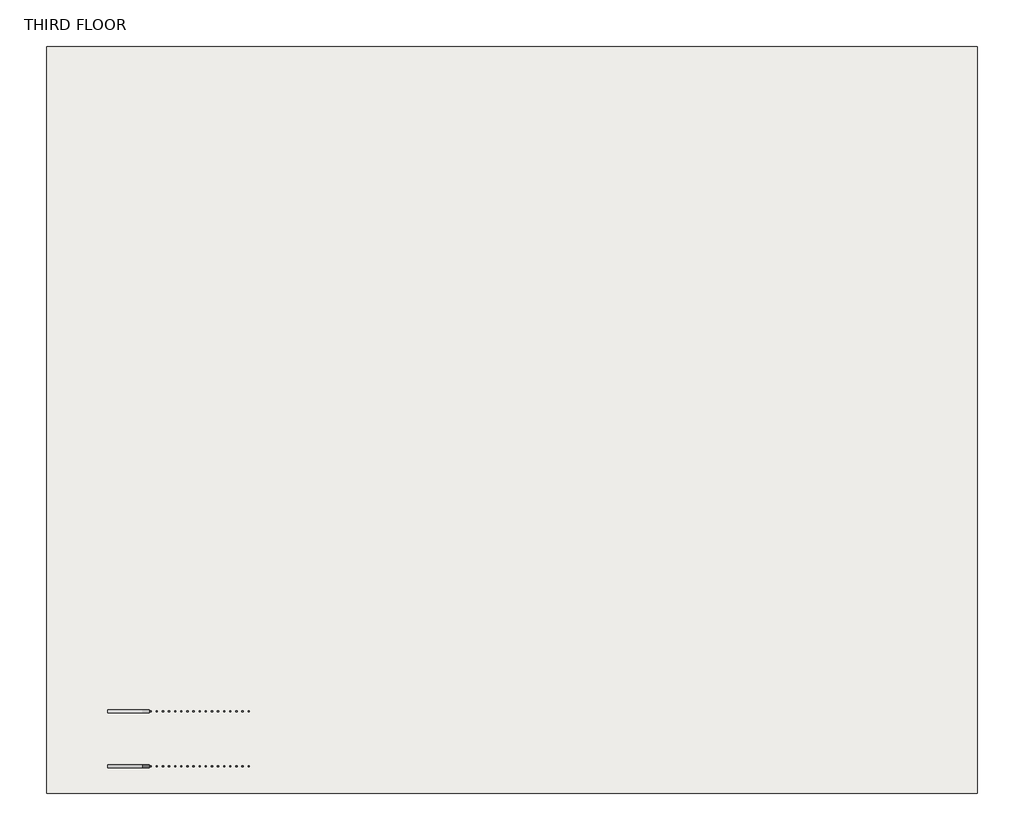
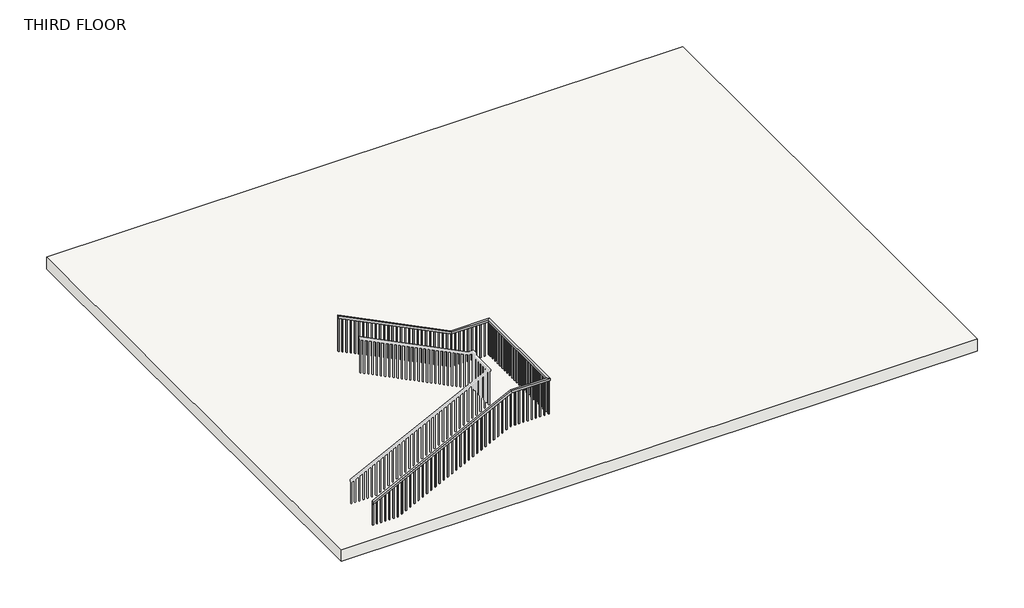
# One storey, part 1 of 2: 1 railing, 1 slab.
"""IFC4 building model written with IfcOpenShell, lengths in millimetres."""

from ifc_helpers import new_model, si_unit, frame, origin, place, context, project, spatial, polyline, outline, extrude, faceted_brep, element, save

model = new_model("IFC4")

# Units and contexts
model_context = context("Model", 3, world=origin())
ifc_project = project(units=[si_unit("LENGTHUNIT", "METRE", prefix="MILLI")], contexts=[model_context])

# Site, building, storey
site = spatial("IfcSite", under=ifc_project)
building = spatial("IfcBuilding", under=site)
storey = spatial("IfcBuildingStorey", under=building, Name="THIRD FLOOR", Elevation=9144.0)

# Railing
placement = place(None, origin())
element("IfcRailing", 1, ObjectType="Handrail - Rectangular", at=placement, inside=storey, context=model_context, shape_type="SolidModel", body=[
    faceted_brep([(-8362.2800418, -5370.1090076, 10058.4), (-8362.2800418, -5370.1090076, 10001.6038734), (-8362.2800418, -5420.9090076, 10001.6038734), (-8362.2800418, -5420.9090076, 10058.4), (-5009.4800418, -5370.1090076, 11734.8), (-4997.4877885, -5370.1090076, 11684.0), (-4997.4877885, -5420.9090076, 11684.0), (-5009.4800418, -5420.9090076, 11734.8), (-4120.4800418, -5370.1090076, 11734.8), (-4120.4800418, -5370.1090076, 11684.0), (-4069.6800418, -5420.9090076, 11684.0), (-4069.6800418, -5420.9090076, 11734.8), (-4120.4800418, -2917.1346494, 11734.8), (-4120.4800418, -2917.1346494, 11684.0), (-4069.6800418, -2866.3346494, 11684.0), (-4069.6800418, -2866.3346494, 11734.8), (-5009.4800418, -2917.1346494, 11734.8), (-5021.472295, -2917.1346494, 11684.0), (-5021.472295, -2866.3346494, 11684.0), (-5009.4800418, -2866.3346494, 11734.8), (-7752.6800418, -2917.1346494, 13106.4), (-7752.6800418, -2866.3346494, 13106.4), (-7752.6800418, -2866.3346494, 13049.6038734), (-7752.6800418, -2917.1346494, 13049.6038734)], [[[0, 1, 2, 3]], [[1, 0, 4, 5]], [[2, 1, 5, 6]], [[3, 2, 6, 7]], [[0, 3, 7, 4]], [[5, 4, 8, 9]], [[6, 5, 9, 10]], [[7, 6, 10, 11]], [[4, 7, 11, 8]], [[9, 8, 12, 13]], [[10, 9, 13, 14]], [[11, 10, 14, 15]], [[8, 11, 15, 12]], [[13, 12, 16, 17]], [[14, 13, 17, 18]], [[15, 14, 18, 19]], [[12, 15, 19, 16]], [[20, 21, 22, 23]], [[17, 16, 20, 23]], [[18, 17, 23, 22]], [[19, 18, 22, 21]], [[16, 19, 21, 20]]]),
    extrude(outline(polyline([(13003.5663734, -7660.6050418), (12145.9625, -7660.6050418), (12136.4375, -7641.5550418), (12994.0413734, -7641.5550418), (13003.5663734, -7660.6050418)])), frame((0.0, -2901.2596494, 0.0), z_axis=(0.0, 1.0, 0.0), x_axis=(0.0, 0.0, 1.0)), (0.0, 0.0, 1.0), 19.05),
    extrude(outline(polyline([(12952.7663734, -7559.0050418), (12095.1625, -7559.0050418), (12085.6375, -7539.9550418), (12943.2413734, -7539.9550418), (12952.7663734, -7559.0050418)])), frame((0.0, -2901.2596494, 0.0), z_axis=(0.0, 1.0, 0.0), x_axis=(0.0, 0.0, 1.0)), (0.0, 0.0, 1.0), 19.05),
    extrude(outline(polyline([(12901.9663734, -7457.4050418), (12044.3625, -7457.4050418), (12034.8375, -7438.3550418), (12892.4413734, -7438.3550418), (12901.9663734, -7457.4050418)])), frame((0.0, -2901.2596494, 0.0), z_axis=(0.0, 1.0, 0.0), x_axis=(0.0, 0.0, 1.0)), (0.0, 0.0, 1.0), 19.05),
    extrude(outline(polyline([(12851.1663734, -7355.8050418), (11993.5625, -7355.8050418), (11984.0375, -7336.7550418), (12841.6413734, -7336.7550418), (12851.1663734, -7355.8050418)])), frame((0.0, -2901.2596494, 0.0), z_axis=(0.0, 1.0, 0.0), x_axis=(0.0, 0.0, 1.0)), (0.0, 0.0, 1.0), 19.05),
    extrude(outline(polyline([(12800.3663734, -7254.2050418), (11942.7625, -7254.2050418), (11933.2375, -7235.1550418), (12790.8413734, -7235.1550418), (12800.3663734, -7254.2050418)])), frame((0.0, -2901.2596494, 0.0), z_axis=(0.0, 1.0, 0.0), x_axis=(0.0, 0.0, 1.0)), (0.0, 0.0, 1.0), 19.05),
    extrude(outline(polyline([(12749.5663734, -7152.6050418), (11891.9625, -7152.6050418), (11882.4375, -7133.5550418), (12740.0413734, -7133.5550418), (12749.5663734, -7152.6050418)])), frame((0.0, -2901.2596494, 0.0), z_axis=(0.0, 1.0, 0.0), x_axis=(0.0, 0.0, 1.0)), (0.0, 0.0, 1.0), 19.05),
    extrude(outline(polyline([(12698.7663734, -7051.0050418), (11841.1625, -7051.0050418), (11831.6375, -7031.9550418), (12689.2413734, -7031.9550418), (12698.7663734, -7051.0050418)])), frame((0.0, -2901.2596494, 0.0), z_axis=(0.0, 1.0, 0.0), x_axis=(0.0, 0.0, 1.0)), (0.0, 0.0, 1.0), 19.05),
    extrude(outline(polyline([(12647.9663734, -6949.4050418), (11790.3625, -6949.4050418), (11780.8375, -6930.3550418), (12638.4413734, -6930.3550418), (12647.9663734, -6949.4050418)])), frame((0.0, -2901.2596494, 0.0), z_axis=(0.0, 1.0, 0.0), x_axis=(0.0, 0.0, 1.0)), (0.0, 0.0, 1.0), 19.05),
    extrude(outline(polyline([(12597.1663734, -6847.8050418), (11739.5625, -6847.8050418), (11730.0375, -6828.7550418), (12587.6413734, -6828.7550418), (12597.1663734, -6847.8050418)])), frame((0.0, -2901.2596494, 0.0), z_axis=(0.0, 1.0, 0.0), x_axis=(0.0, 0.0, 1.0)), (0.0, 0.0, 1.0), 19.05),
    extrude(outline(polyline([(12546.3663734, -6746.2050418), (11688.7625, -6746.2050418), (11679.2375, -6727.1550418), (12536.8413734, -6727.1550418), (12546.3663734, -6746.2050418)])), frame((0.0, -2901.2596494, 0.0), z_axis=(0.0, 1.0, 0.0), x_axis=(0.0, 0.0, 1.0)), (0.0, 0.0, 1.0), 19.05),
    extrude(outline(polyline([(12495.5663734, -6644.6050418), (11637.9625, -6644.6050418), (11628.4375, -6625.5550418), (12486.0413734, -6625.5550418), (12495.5663734, -6644.6050418)])), frame((0.0, -2901.2596494, 0.0), z_axis=(0.0, 1.0, 0.0), x_axis=(0.0, 0.0, 1.0)), (0.0, 0.0, 1.0), 19.05),
    extrude(outline(polyline([(12444.7663734, -6543.0050418), (11587.1625, -6543.0050418), (11577.6375, -6523.9550418), (12435.2413734, -6523.9550418), (12444.7663734, -6543.0050418)])), frame((0.0, -2901.2596494, 0.0), z_axis=(0.0, 1.0, 0.0), x_axis=(0.0, 0.0, 1.0)), (0.0, 0.0, 1.0), 19.05),
    extrude(outline(polyline([(12393.9663734, -6441.4050418), (11536.3625, -6441.4050418), (11526.8375, -6422.3550418), (12384.4413734, -6422.3550418), (12393.9663734, -6441.4050418)])), frame((0.0, -2901.2596494, 0.0), z_axis=(0.0, 1.0, 0.0), x_axis=(0.0, 0.0, 1.0)), (0.0, 0.0, 1.0), 19.05),
    extrude(outline(polyline([(12343.1663734, -6339.8050418), (11485.5625, -6339.8050418), (11476.0375, -6320.7550418), (12333.6413734, -6320.7550418), (12343.1663734, -6339.8050418)])), frame((0.0, -2901.2596494, 0.0), z_axis=(0.0, 1.0, 0.0), x_axis=(0.0, 0.0, 1.0)), (0.0, 0.0, 1.0), 19.05),
    extrude(outline(polyline([(12292.3663734, -6238.2050418), (11434.7625, -6238.2050418), (11425.2375, -6219.1550418), (12282.8413734, -6219.1550418), (12292.3663734, -6238.2050418)])), frame((0.0, -2901.2596494, 0.0), z_axis=(0.0, 1.0, 0.0), x_axis=(0.0, 0.0, 1.0)), (0.0, 0.0, 1.0), 19.05),
    extrude(outline(polyline([(12241.5663734, -6136.6050418), (11383.9625, -6136.6050418), (11374.4375, -6117.5550418), (12232.0413734, -6117.5550418), (12241.5663734, -6136.6050418)])), frame((0.0, -2901.2596494, 0.0), z_axis=(0.0, 1.0, 0.0), x_axis=(0.0, 0.0, 1.0)), (0.0, 0.0, 1.0), 19.05),
    extrude(outline(polyline([(12190.7663734, -6035.0050418), (11333.1625, -6035.0050418), (11323.6375, -6015.9550418), (12181.2413734, -6015.9550418), (12190.7663734, -6035.0050418)])), frame((0.0, -2901.2596494, 0.0), z_axis=(0.0, 1.0, 0.0), x_axis=(0.0, 0.0, 1.0)), (0.0, 0.0, 1.0), 19.05),
    extrude(outline(polyline([(12139.9663734, -5933.4050418), (11282.3625, -5933.4050418), (11272.8375, -5914.3550418), (12130.4413734, -5914.3550418), (12139.9663734, -5933.4050418)])), frame((0.0, -2901.2596494, 0.0), z_axis=(0.0, 1.0, 0.0), x_axis=(0.0, 0.0, 1.0)), (0.0, 0.0, 1.0), 19.05),
    extrude(outline(polyline([(12089.1663734, -5831.8050418), (11231.5625, -5831.8050418), (11222.0375, -5812.7550418), (12079.6413734, -5812.7550418), (12089.1663734, -5831.8050418)])), frame((0.0, -2901.2596494, 0.0), z_axis=(0.0, 1.0, 0.0), x_axis=(0.0, 0.0, 1.0)), (0.0, 0.0, 1.0), 19.05),
    extrude(outline(polyline([(12038.3663734, -5730.2050418), (11180.7625, -5730.2050418), (11171.2375, -5711.1550418), (12028.8413734, -5711.1550418), (12038.3663734, -5730.2050418)])), frame((0.0, -2901.2596494, 0.0), z_axis=(0.0, 1.0, 0.0), x_axis=(0.0, 0.0, 1.0)), (0.0, 0.0, 1.0), 19.05),
    extrude(outline(polyline([(11987.5663734, -5628.6050418), (11129.9625, -5628.6050418), (11120.4375, -5609.5550418), (11978.0413734, -5609.5550418), (11987.5663734, -5628.6050418)])), frame((0.0, -2901.2596494, 0.0), z_axis=(0.0, 1.0, 0.0), x_axis=(0.0, 0.0, 1.0)), (0.0, 0.0, 1.0), 19.05),
    extrude(outline(polyline([(11936.7663734, -5527.0050418), (11079.1625, -5527.0050418), (11069.6375, -5507.9550418), (11927.2413734, -5507.9550418), (11936.7663734, -5527.0050418)])), frame((0.0, -2901.2596494, 0.0), z_axis=(0.0, 1.0, 0.0), x_axis=(0.0, 0.0, 1.0)), (0.0, 0.0, 1.0), 19.05),
    extrude(outline(polyline([(11885.9663734, -5425.4050418), (11028.3625, -5425.4050418), (11018.8375, -5406.3550418), (11876.4413734, -5406.3550418), (11885.9663734, -5425.4050418)])), frame((0.0, -2901.2596494, 0.0), z_axis=(0.0, 1.0, 0.0), x_axis=(0.0, 0.0, 1.0)), (0.0, 0.0, 1.0), 19.05),
    extrude(outline(polyline([(11835.1663734, -5323.8050418), (10977.5625, -5323.8050418), (10968.0375, -5304.7550418), (11825.6413734, -5304.7550418), (11835.1663734, -5323.8050418)])), frame((0.0, -2901.2596494, 0.0), z_axis=(0.0, 1.0, 0.0), x_axis=(0.0, 0.0, 1.0)), (0.0, 0.0, 1.0), 19.05),
    extrude(outline(polyline([(11784.3663734, -5222.2050418), (10926.7625, -5222.2050418), (10917.2375, -5203.1550418), (11774.8413734, -5203.1550418), (11784.3663734, -5222.2050418)])), frame((0.0, -2901.2596494, 0.0), z_axis=(0.0, 1.0, 0.0), x_axis=(0.0, 0.0, 1.0)), (0.0, 0.0, 1.0), 19.05),
    extrude(outline(polyline([(11733.5663734, -5120.6050418), (10875.9625, -5120.6050418), (10866.4375, -5101.5550418), (11724.0413734, -5101.5550418), (11733.5663734, -5120.6050418)])), frame((0.0, -2901.2596494, 0.0), z_axis=(0.0, 1.0, 0.0), x_axis=(0.0, 0.0, 1.0)), (0.0, 0.0, 1.0), 19.05),
    extrude(outline(polyline([(-4898.3550418, -2901.2596494), (-4917.4050418, -2901.2596494), (-4917.4050418, -2882.2096494), (-4898.3550418, -2882.2096494), (-4898.3550418, -2901.2596494)])), frame((0.0, 0.0, 10820.4), z_axis=(0.0, 0.0, 1.0), x_axis=(1.0, 0.0, 0.0)), (0.0, 0.0, 1.0), 863.6),
    extrude(outline(polyline([(-4796.7550418, -2901.2596494), (-4815.8050418, -2901.2596494), (-4815.8050418, -2882.2096494), (-4796.7550418, -2882.2096494), (-4796.7550418, -2901.2596494)])), frame((0.0, 0.0, 10820.4), z_axis=(0.0, 0.0, 1.0), x_axis=(1.0, 0.0, 0.0)), (0.0, 0.0, 1.0), 863.6),
    extrude(outline(polyline([(-4695.1550418, -2901.2596494), (-4714.2050418, -2901.2596494), (-4714.2050418, -2882.2096494), (-4695.1550418, -2882.2096494), (-4695.1550418, -2901.2596494)])), frame((0.0, 0.0, 10820.4), z_axis=(0.0, 0.0, 1.0), x_axis=(1.0, 0.0, 0.0)), (0.0, 0.0, 1.0), 863.6),
    extrude(outline(polyline([(-4593.5550418, -2901.2596494), (-4612.6050418, -2901.2596494), (-4612.6050418, -2882.2096494), (-4593.5550418, -2882.2096494), (-4593.5550418, -2901.2596494)])), frame((0.0, 0.0, 10820.4), z_axis=(0.0, 0.0, 1.0), x_axis=(1.0, 0.0, 0.0)), (0.0, 0.0, 1.0), 863.6),
    extrude(outline(polyline([(-4491.9550418, -2901.2596494), (-4511.0050418, -2901.2596494), (-4511.0050418, -2882.2096494), (-4491.9550418, -2882.2096494), (-4491.9550418, -2901.2596494)])), frame((0.0, 0.0, 10820.4), z_axis=(0.0, 0.0, 1.0), x_axis=(1.0, 0.0, 0.0)), (0.0, 0.0, 1.0), 863.6),
    extrude(outline(polyline([(-4390.3550418, -2901.2596494), (-4409.4050418, -2901.2596494), (-4409.4050418, -2882.2096494), (-4390.3550418, -2882.2096494), (-4390.3550418, -2901.2596494)])), frame((0.0, 0.0, 10820.4), z_axis=(0.0, 0.0, 1.0), x_axis=(1.0, 0.0, 0.0)), (0.0, 0.0, 1.0), 863.6),
    extrude(outline(polyline([(-4288.7550418, -2901.2596494), (-4307.8050418, -2901.2596494), (-4307.8050418, -2882.2096494), (-4288.7550418, -2882.2096494), (-4288.7550418, -2901.2596494)])), frame((0.0, 0.0, 10820.4), z_axis=(0.0, 0.0, 1.0), x_axis=(1.0, 0.0, 0.0)), (0.0, 0.0, 1.0), 863.6),
    extrude(outline(polyline([(-4187.1550418, -2901.2596494), (-4206.2050418, -2901.2596494), (-4206.2050418, -2882.2096494), (-4187.1550418, -2882.2096494), (-4187.1550418, -2901.2596494)])), frame((0.0, 0.0, 10820.4), z_axis=(0.0, 0.0, 1.0), x_axis=(1.0, 0.0, 0.0)), (0.0, 0.0, 1.0), 863.6),
    extrude(outline(polyline([(-4104.6050418, -2966.6340076), (-4104.6050418, -2947.5840076), (-4085.5550418, -2947.5840076), (-4085.5550418, -2966.6340076), (-4104.6050418, -2966.6340076)])), frame((0.0, 0.0, 10820.4), z_axis=(0.0, 0.0, 1.0), x_axis=(1.0, 0.0, 0.0)), (0.0, 0.0, 1.0), 863.6),
    extrude(outline(polyline([(-4104.6050418, -3068.2340076), (-4104.6050418, -3049.1840076), (-4085.5550418, -3049.1840076), (-4085.5550418, -3068.2340076), (-4104.6050418, -3068.2340076)])), frame((0.0, 0.0, 10820.4), z_axis=(0.0, 0.0, 1.0), x_axis=(1.0, 0.0, 0.0)), (0.0, 0.0, 1.0), 863.6),
    extrude(outline(polyline([(-4104.6050418, -3169.8340076), (-4104.6050418, -3150.7840076), (-4085.5550418, -3150.7840076), (-4085.5550418, -3169.8340076), (-4104.6050418, -3169.8340076)])), frame((0.0, 0.0, 10820.4), z_axis=(0.0, 0.0, 1.0), x_axis=(1.0, 0.0, 0.0)), (0.0, 0.0, 1.0), 863.6),
    extrude(outline(polyline([(-4104.6050418, -3271.4340076), (-4104.6050418, -3252.3840076), (-4085.5550418, -3252.3840076), (-4085.5550418, -3271.4340076), (-4104.6050418, -3271.4340076)])), frame((0.0, 0.0, 10820.4), z_axis=(0.0, 0.0, 1.0), x_axis=(1.0, 0.0, 0.0)), (0.0, 0.0, 1.0), 863.6),
    extrude(outline(polyline([(-4104.6050418, -3373.0340076), (-4104.6050418, -3353.9840076), (-4085.5550418, -3353.9840076), (-4085.5550418, -3373.0340076), (-4104.6050418, -3373.0340076)])), frame((0.0, 0.0, 10820.4), z_axis=(0.0, 0.0, 1.0), x_axis=(1.0, 0.0, 0.0)), (0.0, 0.0, 1.0), 863.6),
    extrude(outline(polyline([(-4104.6050418, -3474.6340076), (-4104.6050418, -3455.5840076), (-4085.5550418, -3455.5840076), (-4085.5550418, -3474.6340076), (-4104.6050418, -3474.6340076)])), frame((0.0, 0.0, 10820.4), z_axis=(0.0, 0.0, 1.0), x_axis=(1.0, 0.0, 0.0)), (0.0, 0.0, 1.0), 863.6),
    extrude(outline(polyline([(-4104.6050418, -3576.2340076), (-4104.6050418, -3557.1840076), (-4085.5550418, -3557.1840076), (-4085.5550418, -3576.2340076), (-4104.6050418, -3576.2340076)])), frame((0.0, 0.0, 10820.4), z_axis=(0.0, 0.0, 1.0), x_axis=(1.0, 0.0, 0.0)), (0.0, 0.0, 1.0), 863.6),
    extrude(outline(polyline([(-4104.6050418, -3677.8340076), (-4104.6050418, -3658.7840076), (-4085.5550418, -3658.7840076), (-4085.5550418, -3677.8340076), (-4104.6050418, -3677.8340076)])), frame((0.0, 0.0, 10820.4), z_axis=(0.0, 0.0, 1.0), x_axis=(1.0, 0.0, 0.0)), (0.0, 0.0, 1.0), 863.6),
    extrude(outline(polyline([(-4104.6050418, -3779.4340076), (-4104.6050418, -3760.3840076), (-4085.5550418, -3760.3840076), (-4085.5550418, -3779.4340076), (-4104.6050418, -3779.4340076)])), frame((0.0, 0.0, 10820.4), z_axis=(0.0, 0.0, 1.0), x_axis=(1.0, 0.0, 0.0)), (0.0, 0.0, 1.0), 863.6),
    extrude(outline(polyline([(-4104.6050418, -3881.0340076), (-4104.6050418, -3861.9840076), (-4085.5550418, -3861.9840076), (-4085.5550418, -3881.0340076), (-4104.6050418, -3881.0340076)])), frame((0.0, 0.0, 10820.4), z_axis=(0.0, 0.0, 1.0), x_axis=(1.0, 0.0, 0.0)), (0.0, 0.0, 1.0), 863.6),
    extrude(outline(polyline([(-4104.6050418, -3982.6340076), (-4104.6050418, -3963.5840076), (-4085.5550418, -3963.5840076), (-4085.5550418, -3982.6340076), (-4104.6050418, -3982.6340076)])), frame((0.0, 0.0, 10820.4), z_axis=(0.0, 0.0, 1.0), x_axis=(1.0, 0.0, 0.0)), (0.0, 0.0, 1.0), 863.6),
    extrude(outline(polyline([(-4104.6050418, -4084.2340076), (-4104.6050418, -4065.1840076), (-4085.5550418, -4065.1840076), (-4085.5550418, -4084.2340076), (-4104.6050418, -4084.2340076)])), frame((0.0, 0.0, 10820.4), z_axis=(0.0, 0.0, 1.0), x_axis=(1.0, 0.0, 0.0)), (0.0, 0.0, 1.0), 863.6),
    extrude(outline(polyline([(-4104.6050418, -4185.8340076), (-4104.6050418, -4166.7840076), (-4085.5550418, -4166.7840076), (-4085.5550418, -4185.8340076), (-4104.6050418, -4185.8340076)])), frame((0.0, 0.0, 10820.4), z_axis=(0.0, 0.0, 1.0), x_axis=(1.0, 0.0, 0.0)), (0.0, 0.0, 1.0), 863.6),
    extrude(outline(polyline([(-4104.6050418, -4287.4340076), (-4104.6050418, -4268.3840076), (-4085.5550418, -4268.3840076), (-4085.5550418, -4287.4340076), (-4104.6050418, -4287.4340076)])), frame((0.0, 0.0, 10820.4), z_axis=(0.0, 0.0, 1.0), x_axis=(1.0, 0.0, 0.0)), (0.0, 0.0, 1.0), 863.6),
    extrude(outline(polyline([(-4104.6050418, -4389.0340076), (-4104.6050418, -4369.9840076), (-4085.5550418, -4369.9840076), (-4085.5550418, -4389.0340076), (-4104.6050418, -4389.0340076)])), frame((0.0, 0.0, 10820.4), z_axis=(0.0, 0.0, 1.0), x_axis=(1.0, 0.0, 0.0)), (0.0, 0.0, 1.0), 863.6),
    extrude(outline(polyline([(-4104.6050418, -4490.6340076), (-4104.6050418, -4471.5840076), (-4085.5550418, -4471.5840076), (-4085.5550418, -4490.6340076), (-4104.6050418, -4490.6340076)])), frame((0.0, 0.0, 10820.4), z_axis=(0.0, 0.0, 1.0), x_axis=(1.0, 0.0, 0.0)), (0.0, 0.0, 1.0), 863.6),
    extrude(outline(polyline([(-4104.6050418, -4592.2340076), (-4104.6050418, -4573.1840076), (-4085.5550418, -4573.1840076), (-4085.5550418, -4592.2340076), (-4104.6050418, -4592.2340076)])), frame((0.0, 0.0, 10820.4), z_axis=(0.0, 0.0, 1.0), x_axis=(1.0, 0.0, 0.0)), (0.0, 0.0, 1.0), 863.6),
    extrude(outline(polyline([(-4104.6050418, -4693.8340076), (-4104.6050418, -4674.7840076), (-4085.5550418, -4674.7840076), (-4085.5550418, -4693.8340076), (-4104.6050418, -4693.8340076)])), frame((0.0, 0.0, 10820.4), z_axis=(0.0, 0.0, 1.0), x_axis=(1.0, 0.0, 0.0)), (0.0, 0.0, 1.0), 863.6),
    extrude(outline(polyline([(-4104.6050418, -4795.4340076), (-4104.6050418, -4776.3840076), (-4085.5550418, -4776.3840076), (-4085.5550418, -4795.4340076), (-4104.6050418, -4795.4340076)])), frame((0.0, 0.0, 10820.4), z_axis=(0.0, 0.0, 1.0), x_axis=(1.0, 0.0, 0.0)), (0.0, 0.0, 1.0), 863.6),
    extrude(outline(polyline([(-4104.6050418, -4897.0340076), (-4104.6050418, -4877.9840076), (-4085.5550418, -4877.9840076), (-4085.5550418, -4897.0340076), (-4104.6050418, -4897.0340076)])), frame((0.0, 0.0, 10820.4), z_axis=(0.0, 0.0, 1.0), x_axis=(1.0, 0.0, 0.0)), (0.0, 0.0, 1.0), 863.6),
    extrude(outline(polyline([(-4104.6050418, -4998.6340076), (-4104.6050418, -4979.5840076), (-4085.5550418, -4979.5840076), (-4085.5550418, -4998.6340076), (-4104.6050418, -4998.6340076)])), frame((0.0, 0.0, 10820.4), z_axis=(0.0, 0.0, 1.0), x_axis=(1.0, 0.0, 0.0)), (0.0, 0.0, 1.0), 863.6),
    extrude(outline(polyline([(-4104.6050418, -5100.2340076), (-4104.6050418, -5081.1840076), (-4085.5550418, -5081.1840076), (-4085.5550418, -5100.2340076), (-4104.6050418, -5100.2340076)])), frame((0.0, 0.0, 10820.4), z_axis=(0.0, 0.0, 1.0), x_axis=(1.0, 0.0, 0.0)), (0.0, 0.0, 1.0), 863.6),
    extrude(outline(polyline([(-4104.6050418, -5201.8340076), (-4104.6050418, -5182.7840076), (-4085.5550418, -5182.7840076), (-4085.5550418, -5201.8340076), (-4104.6050418, -5201.8340076)])), frame((0.0, 0.0, 10820.4), z_axis=(0.0, 0.0, 1.0), x_axis=(1.0, 0.0, 0.0)), (0.0, 0.0, 1.0), 863.6),
    extrude(outline(polyline([(-4104.6050418, -5303.4340076), (-4104.6050418, -5284.3840076), (-4085.5550418, -5284.3840076), (-4085.5550418, -5303.4340076), (-4104.6050418, -5303.4340076)])), frame((0.0, 0.0, 10820.4), z_axis=(0.0, 0.0, 1.0), x_axis=(1.0, 0.0, 0.0)), (0.0, 0.0, 1.0), 863.6),
    extrude(outline(polyline([(-4206.2050418, -5385.9840076), (-4187.1550418, -5385.9840076), (-4187.1550418, -5405.0340076), (-4206.2050418, -5405.0340076), (-4206.2050418, -5385.9840076)])), frame((0.0, 0.0, 10820.4), z_axis=(0.0, 0.0, 1.0), x_axis=(1.0, 0.0, 0.0)), (0.0, 0.0, 1.0), 863.6),
    extrude(outline(polyline([(-4307.8050418, -5385.9840076), (-4288.7550418, -5385.9840076), (-4288.7550418, -5405.0340076), (-4307.8050418, -5405.0340076), (-4307.8050418, -5385.9840076)])), frame((0.0, 0.0, 10820.4), z_axis=(0.0, 0.0, 1.0), x_axis=(1.0, 0.0, 0.0)), (0.0, 0.0, 1.0), 863.6),
    extrude(outline(polyline([(-4409.4050418, -5385.9840076), (-4390.3550418, -5385.9840076), (-4390.3550418, -5405.0340076), (-4409.4050418, -5405.0340076), (-4409.4050418, -5385.9840076)])), frame((0.0, 0.0, 10820.4), z_axis=(0.0, 0.0, 1.0), x_axis=(1.0, 0.0, 0.0)), (0.0, 0.0, 1.0), 863.6),
    extrude(outline(polyline([(-4511.0050418, -5385.9840076), (-4491.9550418, -5385.9840076), (-4491.9550418, -5405.0340076), (-4511.0050418, -5405.0340076), (-4511.0050418, -5385.9840076)])), frame((0.0, 0.0, 10820.4), z_axis=(0.0, 0.0, 1.0), x_axis=(1.0, 0.0, 0.0)), (0.0, 0.0, 1.0), 863.6),
    extrude(outline(polyline([(-4612.6050418, -5385.9840076), (-4593.5550418, -5385.9840076), (-4593.5550418, -5405.0340076), (-4612.6050418, -5405.0340076), (-4612.6050418, -5385.9840076)])), frame((0.0, 0.0, 10820.4), z_axis=(0.0, 0.0, 1.0), x_axis=(1.0, 0.0, 0.0)), (0.0, 0.0, 1.0), 863.6),
    extrude(outline(polyline([(-4714.2050418, -5385.9840076), (-4695.1550418, -5385.9840076), (-4695.1550418, -5405.0340076), (-4714.2050418, -5405.0340076), (-4714.2050418, -5385.9840076)])), frame((0.0, 0.0, 10820.4), z_axis=(0.0, 0.0, 1.0), x_axis=(1.0, 0.0, 0.0)), (0.0, 0.0, 1.0), 863.6),
    extrude(outline(polyline([(-4815.8050418, -5385.9840076), (-4796.7550418, -5385.9840076), (-4796.7550418, -5405.0340076), (-4815.8050418, -5405.0340076), (-4815.8050418, -5385.9840076)])), frame((0.0, 0.0, 10820.4), z_axis=(0.0, 0.0, 1.0), x_axis=(1.0, 0.0, 0.0)), (0.0, 0.0, 1.0), 863.6),
    extrude(outline(polyline([(-4917.4050418, -5385.9840076), (-4898.3550418, -5385.9840076), (-4898.3550418, -5405.0340076), (-4917.4050418, -5405.0340076), (-4917.4050418, -5385.9840076)])), frame((0.0, 0.0, 10820.4), z_axis=(0.0, 0.0, 1.0), x_axis=(1.0, 0.0, 0.0)), (0.0, 0.0, 1.0), 863.6),
    extrude(outline(polyline([(11622.4413734, -5120.6050418), (10764.8375, -5120.6050418), (10774.3625, -5101.5550418), (11631.9663734, -5101.5550418), (11622.4413734, -5120.6050418)])), frame((0.0, -5405.0340076, 0.0), z_axis=(0.0, 1.0, 0.0), x_axis=(0.0, 0.0, 1.0)), (0.0, 0.0, 1.0), 19.05),
    extrude(outline(polyline([(11571.6413734, -5222.2050418), (10714.0375, -5222.2050418), (10723.5625, -5203.1550418), (11581.1663734, -5203.1550418), (11571.6413734, -5222.2050418)])), frame((0.0, -5405.0340076, 0.0), z_axis=(0.0, 1.0, 0.0), x_axis=(0.0, 0.0, 1.0)), (0.0, 0.0, 1.0), 19.05),
    extrude(outline(polyline([(11520.8413734, -5323.8050418), (10663.2375, -5323.8050418), (10672.7625, -5304.7550418), (11530.3663734, -5304.7550418), (11520.8413734, -5323.8050418)])), frame((0.0, -5405.0340076, 0.0), z_axis=(0.0, 1.0, 0.0), x_axis=(0.0, 0.0, 1.0)), (0.0, 0.0, 1.0), 19.05),
    extrude(outline(polyline([(11470.0413734, -5425.4050418), (10612.4375, -5425.4050418), (10621.9625, -5406.3550418), (11479.5663734, -5406.3550418), (11470.0413734, -5425.4050418)])), frame((0.0, -5405.0340076, 0.0), z_axis=(0.0, 1.0, 0.0), x_axis=(0.0, 0.0, 1.0)), (0.0, 0.0, 1.0), 19.05),
    extrude(outline(polyline([(11419.2413734, -5527.0050418), (10561.6375, -5527.0050418), (10571.1625, -5507.9550418), (11428.7663734, -5507.9550418), (11419.2413734, -5527.0050418)])), frame((0.0, -5405.0340076, 0.0), z_axis=(0.0, 1.0, 0.0), x_axis=(0.0, 0.0, 1.0)), (0.0, 0.0, 1.0), 19.05),
    extrude(outline(polyline([(11368.4413734, -5628.6050418), (10510.8375, -5628.6050418), (10520.3625, -5609.5550418), (11377.9663734, -5609.5550418), (11368.4413734, -5628.6050418)])), frame((0.0, -5405.0340076, 0.0), z_axis=(0.0, 1.0, 0.0), x_axis=(0.0, 0.0, 1.0)), (0.0, 0.0, 1.0), 19.05),
    extrude(outline(polyline([(11317.6413734, -5730.2050418), (10460.0375, -5730.2050418), (10469.5625, -5711.1550418), (11327.1663734, -5711.1550418), (11317.6413734, -5730.2050418)])), frame((0.0, -5405.0340076, 0.0), z_axis=(0.0, 1.0, 0.0), x_axis=(0.0, 0.0, 1.0)), (0.0, 0.0, 1.0), 19.05),
    extrude(outline(polyline([(11266.8413734, -5831.8050418), (10409.2375, -5831.8050418), (10418.7625, -5812.7550418), (11276.3663734, -5812.7550418), (11266.8413734, -5831.8050418)])), frame((0.0, -5405.0340076, 0.0), z_axis=(0.0, 1.0, 0.0), x_axis=(0.0, 0.0, 1.0)), (0.0, 0.0, 1.0), 19.05),
    extrude(outline(polyline([(11216.0413734, -5933.4050418), (10358.4375, -5933.4050418), (10367.9625, -5914.3550418), (11225.5663734, -5914.3550418), (11216.0413734, -5933.4050418)])), frame((0.0, -5405.0340076, 0.0), z_axis=(0.0, 1.0, 0.0), x_axis=(0.0, 0.0, 1.0)), (0.0, 0.0, 1.0), 19.05),
    extrude(outline(polyline([(11165.2413734, -6035.0050418), (10307.6375, -6035.0050418), (10317.1625, -6015.9550418), (11174.7663734, -6015.9550418), (11165.2413734, -6035.0050418)])), frame((0.0, -5405.0340076, 0.0), z_axis=(0.0, 1.0, 0.0), x_axis=(0.0, 0.0, 1.0)), (0.0, 0.0, 1.0), 19.05),
    extrude(outline(polyline([(11114.4413734, -6136.6050418), (10256.8375, -6136.6050418), (10266.3625, -6117.5550418), (11123.9663734, -6117.5550418), (11114.4413734, -6136.6050418)])), frame((0.0, -5405.0340076, 0.0), z_axis=(0.0, 1.0, 0.0), x_axis=(0.0, 0.0, 1.0)), (0.0, 0.0, 1.0), 19.05),
    extrude(outline(polyline([(11063.6413734, -6238.2050418), (10206.0375, -6238.2050418), (10215.5625, -6219.1550418), (11073.1663734, -6219.1550418), (11063.6413734, -6238.2050418)])), frame((0.0, -5405.0340076, 0.0), z_axis=(0.0, 1.0, 0.0), x_axis=(0.0, 0.0, 1.0)), (0.0, 0.0, 1.0), 19.05),
    extrude(outline(polyline([(11012.8413734, -6339.8050418), (10155.2375, -6339.8050418), (10164.7625, -6320.7550418), (11022.3663734, -6320.7550418), (11012.8413734, -6339.8050418)])), frame((0.0, -5405.0340076, 0.0), z_axis=(0.0, 1.0, 0.0), x_axis=(0.0, 0.0, 1.0)), (0.0, 0.0, 1.0), 19.05),
    extrude(outline(polyline([(10962.0413734, -6441.4050418), (10104.4375, -6441.4050418), (10113.9625, -6422.3550418), (10971.5663734, -6422.3550418), (10962.0413734, -6441.4050418)])), frame((0.0, -5405.0340076, 0.0), z_axis=(0.0, 1.0, 0.0), x_axis=(0.0, 0.0, 1.0)), (0.0, 0.0, 1.0), 19.05),
    extrude(outline(polyline([(10911.2413734, -6543.0050418), (10053.6375, -6543.0050418), (10063.1625, -6523.9550418), (10920.7663734, -6523.9550418), (10911.2413734, -6543.0050418)])), frame((0.0, -5405.0340076, 0.0), z_axis=(0.0, 1.0, 0.0), x_axis=(0.0, 0.0, 1.0)), (0.0, 0.0, 1.0), 19.05),
    extrude(outline(polyline([(10860.4413734, -6644.6050418), (10002.8375, -6644.6050418), (10012.3625, -6625.5550418), (10869.9663734, -6625.5550418), (10860.4413734, -6644.6050418)])), frame((0.0, -5405.0340076, 0.0), z_axis=(0.0, 1.0, 0.0), x_axis=(0.0, 0.0, 1.0)), (0.0, 0.0, 1.0), 19.05),
    extrude(outline(polyline([(10809.6413734, -6746.2050418), (9952.0375, -6746.2050418), (9961.5625, -6727.1550418), (10819.1663734, -6727.1550418), (10809.6413734, -6746.2050418)])), frame((0.0, -5405.0340076, 0.0), z_axis=(0.0, 1.0, 0.0), x_axis=(0.0, 0.0, 1.0)), (0.0, 0.0, 1.0), 19.05),
    extrude(outline(polyline([(10758.8413734, -6847.8050418), (9901.2375, -6847.8050418), (9910.7625, -6828.7550418), (10768.3663734, -6828.7550418), (10758.8413734, -6847.8050418)])), frame((0.0, -5405.0340076, 0.0), z_axis=(0.0, 1.0, 0.0), x_axis=(0.0, 0.0, 1.0)), (0.0, 0.0, 1.0), 19.05),
    extrude(outline(polyline([(10708.0413734, -6949.4050418), (9850.4375, -6949.4050418), (9859.9625, -6930.3550418), (10717.5663734, -6930.3550418), (10708.0413734, -6949.4050418)])), frame((0.0, -5405.0340076, 0.0), z_axis=(0.0, 1.0, 0.0), x_axis=(0.0, 0.0, 1.0)), (0.0, 0.0, 1.0), 19.05),
    extrude(outline(polyline([(10657.2413734, -7051.0050418), (9799.6375, -7051.0050418), (9809.1625, -7031.9550418), (10666.7663734, -7031.9550418), (10657.2413734, -7051.0050418)])), frame((0.0, -5405.0340076, 0.0), z_axis=(0.0, 1.0, 0.0), x_axis=(0.0, 0.0, 1.0)), (0.0, 0.0, 1.0), 19.05),
    extrude(outline(polyline([(10606.4413734, -7152.6050418), (9748.8375, -7152.6050418), (9758.3625, -7133.5550418), (10615.9663734, -7133.5550418), (10606.4413734, -7152.6050418)])), frame((0.0, -5405.0340076, 0.0), z_axis=(0.0, 1.0, 0.0), x_axis=(0.0, 0.0, 1.0)), (0.0, 0.0, 1.0), 19.05),
    extrude(outline(polyline([(10555.6413734, -7254.2050418), (9698.0375, -7254.2050418), (9707.5625, -7235.1550418), (10565.1663734, -7235.1550418), (10555.6413734, -7254.2050418)])), frame((0.0, -5405.0340076, 0.0), z_axis=(0.0, 1.0, 0.0), x_axis=(0.0, 0.0, 1.0)), (0.0, 0.0, 1.0), 19.05),
    extrude(outline(polyline([(10504.8413734, -7355.8050418), (9647.2375, -7355.8050418), (9656.7625, -7336.7550418), (10514.3663734, -7336.7550418), (10504.8413734, -7355.8050418)])), frame((0.0, -5405.0340076, 0.0), z_axis=(0.0, 1.0, 0.0), x_axis=(0.0, 0.0, 1.0)), (0.0, 0.0, 1.0), 19.05),
    extrude(outline(polyline([(10454.0413734, -7457.4050418), (9596.4375, -7457.4050418), (9605.9625, -7438.3550418), (10463.5663734, -7438.3550418), (10454.0413734, -7457.4050418)])), frame((0.0, -5405.0340076, 0.0), z_axis=(0.0, 1.0, 0.0), x_axis=(0.0, 0.0, 1.0)), (0.0, 0.0, 1.0), 19.05),
    extrude(outline(polyline([(10403.2413734, -7559.0050418), (9545.6375, -7559.0050418), (9555.1625, -7539.9550418), (10412.7663734, -7539.9550418), (10403.2413734, -7559.0050418)])), frame((0.0, -5405.0340076, 0.0), z_axis=(0.0, 1.0, 0.0), x_axis=(0.0, 0.0, 1.0)), (0.0, 0.0, 1.0), 19.05),
    extrude(outline(polyline([(10352.4413734, -7660.6050418), (9494.8375, -7660.6050418), (9504.3625, -7641.5550418), (10361.9663734, -7641.5550418), (10352.4413734, -7660.6050418)])), frame((0.0, -5405.0340076, 0.0), z_axis=(0.0, 1.0, 0.0), x_axis=(0.0, 0.0, 1.0)), (0.0, 0.0, 1.0), 19.05),
    extrude(outline(polyline([(10301.6413734, -7762.2050418), (9444.0375, -7762.2050418), (9453.5625, -7743.1550418), (10311.1663734, -7743.1550418), (10301.6413734, -7762.2050418)])), frame((0.0, -5405.0340076, 0.0), z_axis=(0.0, 1.0, 0.0), x_axis=(0.0, 0.0, 1.0)), (0.0, 0.0, 1.0), 19.05),
    extrude(outline(polyline([(10250.8413734, -7863.8050418), (9393.2375, -7863.8050418), (9402.7625, -7844.7550418), (10260.3663734, -7844.7550418), (10250.8413734, -7863.8050418)])), frame((0.0, -5405.0340076, 0.0), z_axis=(0.0, 1.0, 0.0), x_axis=(0.0, 0.0, 1.0)), (0.0, 0.0, 1.0), 19.05),
    extrude(outline(polyline([(10200.0413734, -7965.4050418), (9342.4375, -7965.4050418), (9351.9625, -7946.3550418), (10209.5663734, -7946.3550418), (10200.0413734, -7965.4050418)])), frame((0.0, -5405.0340076, 0.0), z_axis=(0.0, 1.0, 0.0), x_axis=(0.0, 0.0, 1.0)), (0.0, 0.0, 1.0), 19.05),
    extrude(outline(polyline([(10149.2413734, -8067.0050418), (9291.6375, -8067.0050418), (9301.1625, -8047.9550418), (10158.7663734, -8047.9550418), (10149.2413734, -8067.0050418)])), frame((0.0, -5405.0340076, 0.0), z_axis=(0.0, 1.0, 0.0), x_axis=(0.0, 0.0, 1.0)), (0.0, 0.0, 1.0), 19.05),
    extrude(outline(polyline([(10098.4413734, -8168.6050418), (9240.8375, -8168.6050418), (9250.3625, -8149.5550418), (10107.9663734, -8149.5550418), (10098.4413734, -8168.6050418)])), frame((0.0, -5405.0340076, 0.0), z_axis=(0.0, 1.0, 0.0), x_axis=(0.0, 0.0, 1.0)), (0.0, 0.0, 1.0), 19.05),
    extrude(outline(polyline([(10047.6413734, -8270.2050418), (9190.0375, -8270.2050418), (9199.5625, -8251.1550418), (10057.1663734, -8251.1550418), (10047.6413734, -8270.2050418)])), frame((0.0, -5405.0340076, 0.0), z_axis=(0.0, 1.0, 0.0), x_axis=(0.0, 0.0, 1.0)), (0.0, 0.0, 1.0), 19.05),
    extrude(outline(polyline([(-4999.9550418, -2901.2596494), (-5019.0050418, -2901.2596494), (-5019.0050418, -2882.2096494), (-4999.9550418, -2882.2096494), (-4999.9550418, -2901.2596494)])), frame((0.0, 0.0, 10820.4), z_axis=(0.0, 0.0, 1.0), x_axis=(1.0, 0.0, 0.0)), (0.0, 0.0, 1.0), 863.6),
    extrude(outline(polyline([(-4104.6050418, -2901.2596494), (-4104.6050418, -2882.2096494), (-4085.5550418, -2882.2096494), (-4085.5550418, -2901.2596494), (-4104.6050418, -2901.2596494)])), frame((0.0, 0.0, 10820.4), z_axis=(0.0, 0.0, 1.0), x_axis=(1.0, 0.0, 0.0)), (0.0, 0.0, 1.0), 863.6),
    extrude(outline(polyline([(-4104.6050418, -5385.9840076), (-4085.5550418, -5385.9840076), (-4085.5550418, -5405.0340076), (-4104.6050418, -5405.0340076), (-4104.6050418, -5385.9840076)])), frame((0.0, 0.0, 10820.4), z_axis=(0.0, 0.0, 1.0), x_axis=(1.0, 0.0, 0.0)), (0.0, 0.0, 1.0), 863.6),
    extrude(outline(polyline([(11673.2413734, -5019.0050418), (10815.6375, -5019.0050418), (10825.1625, -4999.9550418), (11682.7663734, -4999.9550418), (11673.2413734, -5019.0050418)])), frame((0.0, -5405.0340076, 0.0), z_axis=(0.0, 1.0, 0.0), x_axis=(0.0, 0.0, 1.0)), (0.0, 0.0, 1.0), 19.05),
    extrude(outline(polyline([(13049.6038734, -7752.6800418), (12192.0, -7752.6800418), (12182.475, -7733.6300418), (13040.0788734, -7733.6300418), (13049.6038734, -7752.6800418)])), frame((0.0, -2901.2596494, 0.0), z_axis=(0.0, 1.0, 0.0), x_axis=(0.0, 0.0, 1.0)), (0.0, 0.0, 1.0), 19.05),
    extrude(outline(polyline([(10001.6038734, -8362.2800418), (9144.0, -8362.2800418), (9153.525, -8343.2300418), (10011.1288734, -8343.2300418), (10001.6038734, -8362.2800418)])), frame((0.0, -5405.0340076, 0.0), z_axis=(0.0, 1.0, 0.0), x_axis=(0.0, 0.0, 1.0)), (0.0, 0.0, 1.0), 19.05),
])

# Slab
element("IfcSlab", 2, ObjectType="Generic - 12\"", at=placement, inside=storey, context=model_context, shape_type="SweptSolid", body=[
    extrude(outline(polyline([(6064.2982466, 6554.3761968), (6064.2982466, -5840.8238032), (-9378.9017534, -5840.8238032), (-9378.9017534, 6554.3761968), (6064.2982466, 6554.3761968)])), frame((0.0, 0.0, 9144.0), z_axis=(0.0, 0.0, 1.0), x_axis=(1.0, 0.0, 0.0)), (0.0, 0.0, 1.0), 304.8),
])

save(model, "model.ifc")

# Revit data of these elements
# Type "Handrail - Rectangular"
#   Assembly Code = "C2010400"
#   built-in parameter 1008612 = 0.0416667 (stored number, unit not read)
#   built-in parameter 1008611 = 0.0416667 (stored number, unit not read)
#   built-in parameter 1008609 = 0.333333 (stored number, unit not read)
#   built-in parameter 1008604 = 0.166667 (stored number, unit not read)
#   built-in parameter 1008603 = 0.166667 (stored number, unit not read)
#   Railing Height = 3' - 0"
#   built-in parameter 1008630 = 2
#   built-in parameter 1008610 = 2
#   built-in parameter 1008618 = Baluster - Square : 3/4"
# Type "Generic - 12\""
#   Assembly Code = "B1010"
#   Function = 0
#   Layers, outside or top first: 1' - 0" no material (function 1)
# Element 1 (IfcRailing, "Handrail - Rectangular")
#   Phase Created = New Construction
# Element 2 (IfcSlab, "Generic - 12\"")
#   Height Offset From Level = 1' - 0"
#   Phase Created = New Construction
#   Materials on its faces: "Default Floor"
# Materials
#   "Default Floor": colour RGB 128 128 128, transparency 0, Cost = 0
